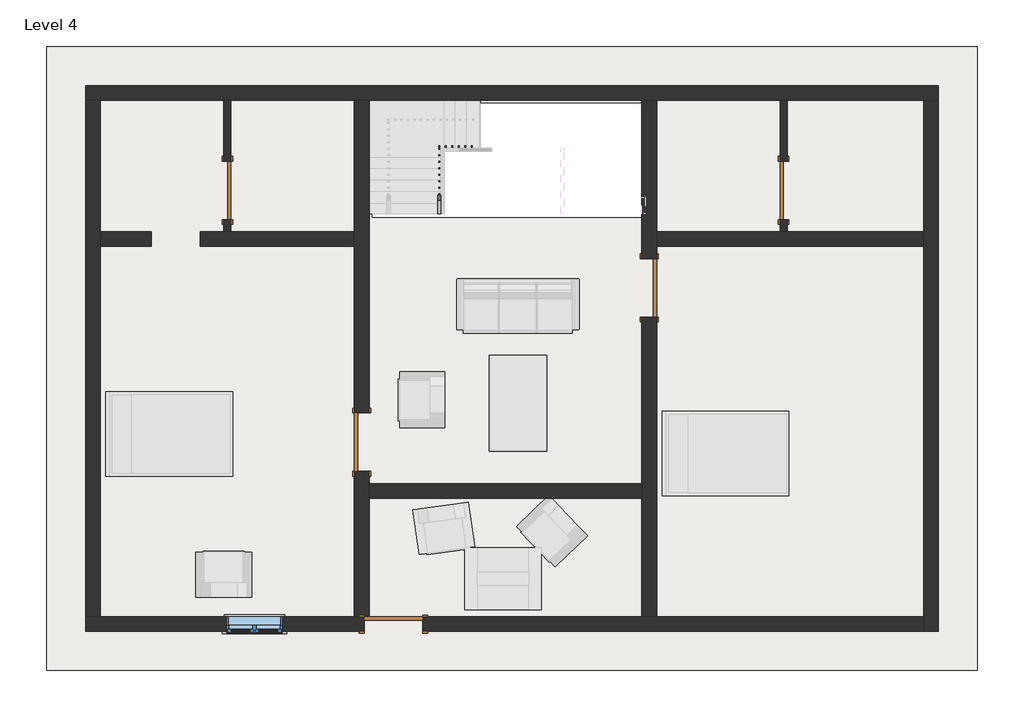
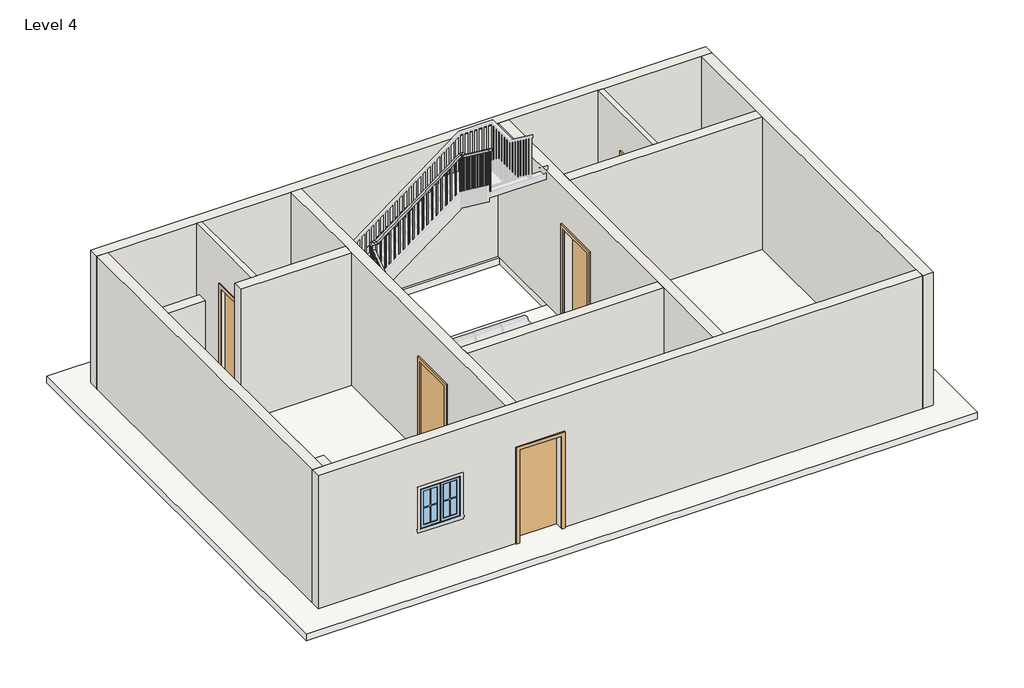
# One storey, part 1 of 2: 12 walls, 5 doors, 1 railing, 1 roof, 1 window.
"""IFC4 building model written with IfcOpenShell, lengths in millimetres."""

from ifc_helpers import new_model, si_unit, frame, origin, place, context, project, spatial, polyline, outline, extrude, faceted_brep, transform, mapped, element, save
from components import door_e5f9f3c4, door_a90ba1ad, door_305aa2a5, window_339605e1

model = new_model("IFC4")

# Units and contexts
model_context = context("Model", 3, world=origin())
ifc_project = project(units=[si_unit("LENGTHUNIT", "METRE", prefix="MILLI")], contexts=[model_context])

# Site, building, storey
site = spatial("IfcSite", under=ifc_project)
building = spatial("IfcBuilding", under=site)
storey = spatial("IfcBuildingStorey", under=building, Name="Level 4", Elevation=6400.8)

# Doors
placement = place(None, origin())
door_shape = door_e5f9f3c4(model_context)
element("IfcDoor", 1, ObjectType="Single-Flush : 36\" x 84\"", at=placement, inside=storey, context=model_context, shape_type="MappedRepresentation", body=[
    mapped(door_shape, transform((-5709.1546642, 5087.2167606, 6400.8), x_axis=(0.0, -1.0, 0.0), y_axis=(1.0, 0.0, 0.0), z_axis=(0.0, 0.0, 1.0))),
])
door_2_shape = door_a90ba1ad(model_context)
element("IfcDoor", 2, ObjectType="Single-Flush : 36\" x 84\"", at=placement, inside=storey, context=model_context, shape_type="MappedRepresentation", body=[
    mapped(door_2_shape, transform((-3607.3046642, 1150.2167606, 6400.8), x_axis=(0.0, -1.0, 0.0), y_axis=(1.0, 0.0, 0.0), z_axis=(0.0, 0.0, 1.0))),
])
element("IfcDoor", 3, ObjectType="Single-Flush : 36\" x 84\"", at=placement, inside=storey, context=model_context, shape_type="MappedRepresentation", body=[
    mapped(door_2_shape, transform((888.4953358, 3563.2167606, 6400.8), x_axis=(0.0, 1.0, 0.0), y_axis=(-1.0, 0.0, 0.0), z_axis=(0.0, 0.0, 1.0))),
])
element("IfcDoor", 4, ObjectType="Single-Flush : 36\" x 84\"", at=placement, inside=storey, context=model_context, shape_type="MappedRepresentation", body=[
    mapped(door_2_shape, transform((-3112.0046642, -1694.5832394, 6400.8), x_axis=(-1.0, 0.0, 0.0), y_axis=(0.0, -1.0, 0.0), z_axis=(0.0, 0.0, 1.0))),
])
door_3_shape = door_305aa2a5(model_context)
element("IfcDoor", 5, ObjectType="Single-Flush : 36\" x 84\"", at=placement, inside=storey, context=model_context, shape_type="MappedRepresentation", body=[
    mapped(door_3_shape, transform((2990.3453358, 5087.2167606, 6400.8), x_axis=(0.0, -1.0, 0.0), y_axis=(1.0, 0.0, 0.0), z_axis=(0.0, 0.0, 1.0))),
])

# Railing
element("IfcRailing", 6, ObjectType="Handrail - Rectangular", at=placement, inside=storey, context=model_context, shape_type="SolidModel", body=[
    faceted_brep([(-2419.4972892, 4718.9167606, 7447.7217391), (-2419.4972892, 4718.9167606, 7384.3634439), (-2368.6972892, 4718.9167606, 7384.3634439), (-2368.6972892, 4718.9167606, 7447.7217391), (-2419.4972892, 5670.3536537, 8156.8672495), (-2419.4972892, 5721.1536537, 8131.3723083), (-2368.6972892, 5721.1536537, 8131.3723083), (-2368.6972892, 5670.3536537, 8156.8672495), (-2419.4972892, 5670.3536537, 8263.6733611), (-2419.4972892, 5721.1536537, 8212.8733611), (-2368.6972892, 5721.1536537, 8212.8733611), (-2368.6972892, 5670.3536537, 8263.6733611), (-2419.4972892, 5797.3536537, 8263.6733611), (-2419.4972892, 5797.3536537, 8212.8733611), (-2368.6972892, 5746.5536537, 8212.8733611), (-2368.6972892, 5746.5536537, 8263.6733611), (-2292.4972892, 5797.3536537, 8263.6733611), (-2275.6482431, 5797.3536537, 8212.8733611), (-2275.6482431, 5746.5536537, 8212.8733611), (-2292.4972892, 5746.5536537, 8263.6733611), (-474.1369697, 5797.3536537, 9618.9729781), (-457.2879235, 5797.3536537, 9568.1729781), (-457.2879235, 5746.5536537, 9568.1729781), (-474.1369697, 5746.5536537, 9618.9729781), (-394.2046642, 5797.3536537, 9618.9729781), (-394.2046642, 5797.3536537, 9568.1729781), (-445.0046642, 5746.5536537, 9568.1729781), (-445.0046642, 5746.5536537, 9618.9729781), (-394.2046642, 5717.4213483, 9618.9729781), (-394.2046642, 5700.5723021, 9568.1729781), (-445.0046642, 5700.5723021, 9568.1729781), (-445.0046642, 5717.4213483, 9618.9729781), (-394.2046642, 4718.9167606, 10363.2), (-445.0046642, 4718.9167606, 10363.2), (-445.0046642, 4718.9167606, 10299.8417047), (-394.2046642, 4718.9167606, 10299.8417047)], [[[0, 1, 2, 3]], [[1, 0, 4, 5]], [[2, 1, 5, 6]], [[3, 2, 6, 7]], [[0, 3, 7, 4]], [[5, 4, 8, 9]], [[6, 5, 9, 10]], [[7, 6, 10, 11]], [[4, 7, 11, 8]], [[9, 8, 12, 13]], [[10, 9, 13, 14]], [[11, 10, 14, 15]], [[8, 11, 15, 12]], [[13, 12, 16, 17]], [[14, 13, 17, 18]], [[15, 14, 18, 19]], [[12, 15, 19, 16]], [[17, 16, 20, 21]], [[18, 17, 21, 22]], [[19, 18, 22, 23]], [[16, 19, 23, 20]], [[21, 20, 24, 25]], [[22, 21, 25, 26]], [[23, 22, 26, 27]], [[20, 23, 27, 24]], [[25, 24, 28, 29]], [[26, 25, 29, 30]], [[27, 26, 30, 31]], [[24, 27, 31, 28]], [[32, 33, 34, 35]], [[29, 28, 32, 35]], [[30, 29, 35, 34]], [[31, 30, 34, 33]], [[28, 31, 33, 32]]]),
    extrude(outline(polyline([(4746.4286537, 10279.3359459), (4765.4786537, 10265.1371882), (4765.4786537, 9316.2782609), (4746.4286537, 9316.2782609), (4746.4286537, 10279.3359459)])), frame((-429.1296642, 0.0, 0.0), z_axis=(1.0, 0.0, 0.0), x_axis=(0.0, 1.0, 0.0)), (0.0, 0.0, 1.0), 19.05),
    extrude(outline(polyline([(4848.0286537, 10203.6092378), (4867.0786537, 10189.4104801), (4867.0786537, 9316.2782609), (4848.0286537, 9316.2782609), (4848.0286537, 10203.6092378)])), frame((-429.1296642, 0.0, 0.0), z_axis=(1.0, 0.0, 0.0), x_axis=(0.0, 1.0, 0.0)), (0.0, 0.0, 1.0), 19.05),
    extrude(outline(polyline([(4949.6286537, 10127.8825298), (4968.6786537, 10113.683772), (4968.6786537, 9183.7565217), (4949.6286537, 9183.7565217), (4949.6286537, 10127.8825298)])), frame((-429.1296642, 0.0, 0.0), z_axis=(1.0, 0.0, 0.0), x_axis=(0.0, 1.0, 0.0)), (0.0, 0.0, 1.0), 19.05),
    extrude(outline(polyline([(5051.2286537, 10052.1558217), (5070.2786537, 10037.9570639), (5070.2786537, 9183.7565217), (5051.2286537, 9183.7565217), (5051.2286537, 10052.1558217)])), frame((-429.1296642, 0.0, 0.0), z_axis=(1.0, 0.0, 0.0), x_axis=(0.0, 1.0, 0.0)), (0.0, 0.0, 1.0), 19.05),
    extrude(outline(polyline([(5152.8286537, 9976.4291136), (5171.8786537, 9962.2303559), (5171.8786537, 9051.2347826), (5152.8286537, 9051.2347826), (5152.8286537, 9976.4291136)])), frame((-429.1296642, 0.0, 0.0), z_axis=(1.0, 0.0, 0.0), x_axis=(0.0, 1.0, 0.0)), (0.0, 0.0, 1.0), 19.05),
    extrude(outline(polyline([(5254.4286537, 9900.7024055), (5273.4786537, 9886.5036478), (5273.4786537, 8918.7130435), (5254.4286537, 8918.7130435), (5254.4286537, 9900.7024055)])), frame((-429.1296642, 0.0, 0.0), z_axis=(1.0, 0.0, 0.0), x_axis=(0.0, 1.0, 0.0)), (0.0, 0.0, 1.0), 19.05),
    extrude(outline(polyline([(5356.0286537, 9824.9756975), (5375.0786537, 9810.7769397), (5375.0786537, 8918.7130435), (5356.0286537, 8918.7130435), (5356.0286537, 9824.9756975)])), frame((-429.1296642, 0.0, 0.0), z_axis=(1.0, 0.0, 0.0), x_axis=(0.0, 1.0, 0.0)), (0.0, 0.0, 1.0), 19.05),
    extrude(outline(polyline([(5457.6286537, 9749.2489894), (5476.6786537, 9735.0502316), (5476.6786537, 8786.1913043), (5457.6286537, 8786.1913043), (5457.6286537, 9749.2489894)])), frame((-429.1296642, 0.0, 0.0), z_axis=(1.0, 0.0, 0.0), x_axis=(0.0, 1.0, 0.0)), (0.0, 0.0, 1.0), 19.05),
    extrude(outline(polyline([(5559.2286537, 9673.5222813), (5578.2786537, 9659.3235236), (5578.2786537, 8786.1913043), (5559.2286537, 8786.1913043), (5559.2286537, 9673.5222813)])), frame((-429.1296642, 0.0, 0.0), z_axis=(1.0, 0.0, 0.0), x_axis=(0.0, 1.0, 0.0)), (0.0, 0.0, 1.0), 19.05),
    extrude(outline(polyline([(5660.8286537, 9597.7955732), (5679.8786537, 9583.5968155), (5679.8786537, 8653.6695652), (5660.8286537, 8653.6695652), (5660.8286537, 9597.7955732)])), frame((-429.1296642, 0.0, 0.0), z_axis=(1.0, 0.0, 0.0), x_axis=(0.0, 1.0, 0.0)), (0.0, 0.0, 1.0), 19.05),
    extrude(outline(polyline([(-473.2222892, 5762.4286537), (-473.2222892, 5781.4786537), (-454.1722892, 5781.4786537), (-454.1722892, 5762.4286537), (-473.2222892, 5762.4286537)])), frame((0.0, 0.0, 8653.6695652), z_axis=(0.0, 0.0, 1.0), x_axis=(1.0, 0.0, 0.0)), (0.0, 0.0, 1.0), 914.5034129),
    extrude(outline(polyline([(9494.7684819, -555.7722892), (9480.5697242, -574.8222892), (8521.1478261, -574.8222892), (8521.1478261, -555.7722892), (9494.7684819, -555.7722892)])), frame((0.0, 5762.4286537, 0.0), z_axis=(0.0, 1.0, 0.0), x_axis=(0.0, 0.0, 1.0)), (0.0, 0.0, 1.0), 19.05),
    extrude(outline(polyline([(9419.0417739, -657.3722892), (9404.8430161, -676.4222892), (8521.1478261, -676.4222892), (8521.1478261, -657.3722892), (9419.0417739, -657.3722892)])), frame((0.0, 5762.4286537, 0.0), z_axis=(0.0, 1.0, 0.0), x_axis=(0.0, 0.0, 1.0)), (0.0, 0.0, 1.0), 19.05),
    extrude(outline(polyline([(9343.3150658, -758.9722892), (9329.116308, -778.0222892), (8388.626087, -778.0222892), (8388.626087, -758.9722892), (9343.3150658, -758.9722892)])), frame((0.0, 5762.4286537, 0.0), z_axis=(0.0, 1.0, 0.0), x_axis=(0.0, 0.0, 1.0)), (0.0, 0.0, 1.0), 19.05),
    extrude(outline(polyline([(9267.5883577, -860.5722892), (9253.3896, -879.6222892), (8388.626087, -879.6222892), (8388.626087, -860.5722892), (9267.5883577, -860.5722892)])), frame((0.0, 5762.4286537, 0.0), z_axis=(0.0, 1.0, 0.0), x_axis=(0.0, 0.0, 1.0)), (0.0, 0.0, 1.0), 19.05),
    extrude(outline(polyline([(9191.8616496, -962.1722892), (9177.6628919, -981.2222892), (8256.1043478, -981.2222892), (8256.1043478, -962.1722892), (9191.8616496, -962.1722892)])), frame((0.0, 5762.4286537, 0.0), z_axis=(0.0, 1.0, 0.0), x_axis=(0.0, 0.0, 1.0)), (0.0, 0.0, 1.0), 19.05),
    extrude(outline(polyline([(9116.1349416, -1063.7722892), (9101.9361838, -1082.8222892), (8256.1043478, -1082.8222892), (8256.1043478, -1063.7722892), (9116.1349416, -1063.7722892)])), frame((0.0, 5762.4286537, 0.0), z_axis=(0.0, 1.0, 0.0), x_axis=(0.0, 0.0, 1.0)), (0.0, 0.0, 1.0), 19.05),
    extrude(outline(polyline([(9040.4082335, -1165.3722892), (9026.2094757, -1184.4222892), (8123.5826087, -1184.4222892), (8123.5826087, -1165.3722892), (9040.4082335, -1165.3722892)])), frame((0.0, 5762.4286537, 0.0), z_axis=(0.0, 1.0, 0.0), x_axis=(0.0, 0.0, 1.0)), (0.0, 0.0, 1.0), 19.05),
    extrude(outline(polyline([(8964.6815254, -1266.9722892), (8950.4827677, -1286.0222892), (7991.0608696, -1286.0222892), (7991.0608696, -1266.9722892), (8964.6815254, -1266.9722892)])), frame((0.0, 5762.4286537, 0.0), z_axis=(0.0, 1.0, 0.0), x_axis=(0.0, 0.0, 1.0)), (0.0, 0.0, 1.0), 19.05),
    extrude(outline(polyline([(8888.9548173, -1368.5722892), (8874.7560596, -1387.6222892), (7991.0608696, -1387.6222892), (7991.0608696, -1368.5722892), (8888.9548173, -1368.5722892)])), frame((0.0, 5762.4286537, 0.0), z_axis=(0.0, 1.0, 0.0), x_axis=(0.0, 0.0, 1.0)), (0.0, 0.0, 1.0), 19.05),
    extrude(outline(polyline([(8813.2281093, -1470.1722892), (8799.0293515, -1489.2222892), (7858.5391304, -1489.2222892), (7858.5391304, -1470.1722892), (8813.2281093, -1470.1722892)])), frame((0.0, 5762.4286537, 0.0), z_axis=(0.0, 1.0, 0.0), x_axis=(0.0, 0.0, 1.0)), (0.0, 0.0, 1.0), 19.05),
    extrude(outline(polyline([(8737.5014012, -1571.7722892), (8723.3026434, -1590.8222892), (7858.5391304, -1590.8222892), (7858.5391304, -1571.7722892), (8737.5014012, -1571.7722892)])), frame((0.0, 5762.4286537, 0.0), z_axis=(0.0, 1.0, 0.0), x_axis=(0.0, 0.0, 1.0)), (0.0, 0.0, 1.0), 19.05),
    extrude(outline(polyline([(8661.7746931, -1673.3722892), (8647.5759354, -1692.4222892), (7726.0173913, -1692.4222892), (7726.0173913, -1673.3722892), (8661.7746931, -1673.3722892)])), frame((0.0, 5762.4286537, 0.0), z_axis=(0.0, 1.0, 0.0), x_axis=(0.0, 0.0, 1.0)), (0.0, 0.0, 1.0), 19.05),
    extrude(outline(polyline([(8586.047985, -1774.9722892), (8571.8492273, -1794.0222892), (7726.0173913, -1794.0222892), (7726.0173913, -1774.9722892), (8586.047985, -1774.9722892)])), frame((0.0, 5762.4286537, 0.0), z_axis=(0.0, 1.0, 0.0), x_axis=(0.0, 0.0, 1.0)), (0.0, 0.0, 1.0), 19.05),
    extrude(outline(polyline([(8510.321277, -1876.5722892), (8496.1225192, -1895.6222892), (7593.4956522, -1895.6222892), (7593.4956522, -1876.5722892), (8510.321277, -1876.5722892)])), frame((0.0, 5762.4286537, 0.0), z_axis=(0.0, 1.0, 0.0), x_axis=(0.0, 0.0, 1.0)), (0.0, 0.0, 1.0), 19.05),
    extrude(outline(polyline([(8434.5945689, -1978.1722892), (8420.3958111, -1997.2222892), (7460.973913, -1997.2222892), (7460.973913, -1978.1722892), (8434.5945689, -1978.1722892)])), frame((0.0, 5762.4286537, 0.0), z_axis=(0.0, 1.0, 0.0), x_axis=(0.0, 0.0, 1.0)), (0.0, 0.0, 1.0), 19.05),
    extrude(outline(polyline([(8358.8678608, -2079.7722892), (8344.6691031, -2098.8222892), (7460.973913, -2098.8222892), (7460.973913, -2079.7722892), (8358.8678608, -2079.7722892)])), frame((0.0, 5762.4286537, 0.0), z_axis=(0.0, 1.0, 0.0), x_axis=(0.0, 0.0, 1.0)), (0.0, 0.0, 1.0), 19.05),
    extrude(outline(polyline([(8283.1411527, -2181.3722892), (8268.942395, -2200.4222892), (7328.4521739, -2200.4222892), (7328.4521739, -2181.3722892), (8283.1411527, -2181.3722892)])), frame((0.0, 5762.4286537, 0.0), z_axis=(0.0, 1.0, 0.0), x_axis=(0.0, 0.0, 1.0)), (0.0, 0.0, 1.0), 19.05),
    extrude(outline(polyline([(8207.4144447, -2282.9722892), (8193.2156869, -2302.0222892), (7328.4521739, -2302.0222892), (7328.4521739, -2282.9722892), (8207.4144447, -2282.9722892)])), frame((0.0, 5762.4286537, 0.0), z_axis=(0.0, 1.0, 0.0), x_axis=(0.0, 0.0, 1.0)), (0.0, 0.0, 1.0), 19.05),
    extrude(outline(polyline([(-2384.5722892, 5725.3917606), (-2403.6222892, 5725.3917606), (-2403.6222892, 5744.4417606), (-2384.5722892, 5744.4417606), (-2384.5722892, 5725.3917606)])), frame((0.0, 0.0, 7195.9304348), z_axis=(0.0, 0.0, 1.0), x_axis=(1.0, 0.0, 0.0)), (0.0, 0.0, 1.0), 1016.9429263),
    extrude(outline(polyline([(5623.7917606, 8058.8044377), (5642.8417606, 8073.0031954), (5642.8417606, 7195.9304348), (5623.7917606, 7195.9304348), (5623.7917606, 8058.8044377)])), frame((-2403.6222892, 0.0, 0.0), z_axis=(1.0, 0.0, 0.0), x_axis=(0.0, 1.0, 0.0)), (0.0, 0.0, 1.0), 19.05),
    extrude(outline(polyline([(5522.1917606, 7983.0777296), (5541.2417606, 7997.2764873), (5541.2417606, 7063.4086957), (5522.1917606, 7063.4086957), (5522.1917606, 7983.0777296)])), frame((-2403.6222892, 0.0, 0.0), z_axis=(1.0, 0.0, 0.0), x_axis=(0.0, 1.0, 0.0)), (0.0, 0.0, 1.0), 19.05),
    extrude(outline(polyline([(5420.5917606, 7907.3510215), (5439.6417606, 7921.5497793), (5439.6417606, 7063.4086957), (5420.5917606, 7063.4086957), (5420.5917606, 7907.3510215)])), frame((-2403.6222892, 0.0, 0.0), z_axis=(1.0, 0.0, 0.0), x_axis=(0.0, 1.0, 0.0)), (0.0, 0.0, 1.0), 19.05),
    extrude(outline(polyline([(5318.9917606, 7831.6243134), (5338.0417606, 7845.8230712), (5338.0417606, 6930.8869565), (5318.9917606, 6930.8869565), (5318.9917606, 7831.6243134)])), frame((-2403.6222892, 0.0, 0.0), z_axis=(1.0, 0.0, 0.0), x_axis=(0.0, 1.0, 0.0)), (0.0, 0.0, 1.0), 19.05),
    extrude(outline(polyline([(5217.3917606, 7755.8976054), (5236.4417606, 7770.0963631), (5236.4417606, 6798.3652174), (5217.3917606, 6798.3652174), (5217.3917606, 7755.8976054)])), frame((-2403.6222892, 0.0, 0.0), z_axis=(1.0, 0.0, 0.0), x_axis=(0.0, 1.0, 0.0)), (0.0, 0.0, 1.0), 19.05),
    extrude(outline(polyline([(5115.7917606, 7680.1708973), (5134.8417606, 7694.369655), (5134.8417606, 6798.3652174), (5115.7917606, 6798.3652174), (5115.7917606, 7680.1708973)])), frame((-2403.6222892, 0.0, 0.0), z_axis=(1.0, 0.0, 0.0), x_axis=(0.0, 1.0, 0.0)), (0.0, 0.0, 1.0), 19.05),
    extrude(outline(polyline([(5014.1917606, 7604.4441892), (5033.2417606, 7618.642947), (5033.2417606, 6665.8434783), (5014.1917606, 6665.8434783), (5014.1917606, 7604.4441892)])), frame((-2403.6222892, 0.0, 0.0), z_axis=(1.0, 0.0, 0.0), x_axis=(0.0, 1.0, 0.0)), (0.0, 0.0, 1.0), 19.05),
    extrude(outline(polyline([(4912.5917606, 7528.7174811), (4931.6417606, 7542.9162389), (4931.6417606, 6665.8434783), (4912.5917606, 6665.8434783), (4912.5917606, 7528.7174811)])), frame((-2403.6222892, 0.0, 0.0), z_axis=(1.0, 0.0, 0.0), x_axis=(0.0, 1.0, 0.0)), (0.0, 0.0, 1.0), 19.05),
    extrude(outline(polyline([(4810.9917606, 7452.9907731), (4830.0417606, 7467.1895308), (4830.0417606, 6533.3217391), (4810.9917606, 6533.3217391), (4810.9917606, 7452.9907731)])), frame((-2403.6222892, 0.0, 0.0), z_axis=(1.0, 0.0, 0.0), x_axis=(0.0, 1.0, 0.0)), (0.0, 0.0, 1.0), 19.05),
    extrude(outline(polyline([(-429.1296642, 5762.4286537), (-429.1296642, 5781.4786537), (-410.0796642, 5781.4786537), (-410.0796642, 5762.4286537), (-429.1296642, 5762.4286537)])), frame((0.0, 0.0, 8653.6695652), z_axis=(0.0, 0.0, 1.0), x_axis=(1.0, 0.0, 0.0)), (0.0, 0.0, 1.0), 914.5034129),
    extrude(outline(polyline([(-2384.5722892, 5762.4286537), (-2403.6222892, 5762.4286537), (-2403.6222892, 5781.4786537), (-2384.5722892, 5781.4786537), (-2384.5722892, 5762.4286537)])), frame((0.0, 0.0, 7195.9304348), z_axis=(0.0, 0.0, 1.0), x_axis=(1.0, 0.0, 0.0)), (0.0, 0.0, 1.0), 1016.9429263),
    extrude(outline(polyline([(4718.9167606, 10299.8417047), (4737.9667606, 10285.642947), (4737.9667606, 9316.2782609), (4718.9167606, 9316.2782609), (4718.9167606, 10299.8417047)])), frame((-429.1296642, 0.0, 0.0), z_axis=(1.0, 0.0, 0.0), x_axis=(0.0, 1.0, 0.0)), (0.0, 0.0, 1.0), 19.05),
    extrude(outline(polyline([(4718.9167606, 7384.3634439), (4737.9667606, 7398.5622016), (4737.9667606, 6533.3217391), (4718.9167606, 6533.3217391), (4718.9167606, 7384.3634439)])), frame((-2403.6222892, 0.0, 0.0), z_axis=(1.0, 0.0, 0.0), x_axis=(0.0, 1.0, 0.0)), (0.0, 0.0, 1.0), 19.05),
])

# Roof
element("IfcRoof", 7, ObjectType="Generic - 12\"", at=placement, inside=storey, context=model_context, shape_type="SweptSolid", body=[
    extrude(outline(polyline([(6019.2953358, 7335.1167606), (6019.2953358, -2418.4832394), (-8534.9046642, -2418.4832394), (-8534.9046642, 7335.1167606), (6019.2953358, 7335.1167606)]), holes=[polyline([(774.1953358, 6446.1167606), (-3442.2046642, 6446.1167606), (-3442.2046642, 4668.1167606), (774.1953358, 4668.1167606), (774.1953358, 6446.1167606)])]), frame((0.0, 0.0, 6248.4), z_axis=(0.0, 0.0, 1.0), x_axis=(1.0, 0.0, 0.0)), (0.0, 0.0, 1.0), 152.4),
])

# Walls
element("IfcWall", 8, ObjectType="WALL4.5\"", at=placement, inside=storey, context=model_context, shape_type="SweptSolid", body=[
    extrude(outline(polyline([(4630.0167606, 8534.4), (4630.0167606, 6400.8), (4439.5167606, 6400.8), (4439.5167606, 9448.8), (6496.9167606, 9448.8), (6496.9167606, 6400.8), (5544.4167606, 6400.8), (5544.4167606, 8534.4), (4630.0167606, 8534.4)])), frame((-5766.3046642, 0.0, 0.0), z_axis=(1.0, 0.0, 0.0), x_axis=(0.0, 1.0, 0.0)), (0.0, 0.0, 1.0), 114.3),
])
element("IfcWall", 9, ObjectType="WALL4.5\"", at=placement, inside=storey, context=model_context, shape_type="SweptSolid", body=[
    extrude(outline(polyline([(4630.0167606, 8534.4), (4630.0167606, 6400.8), (4439.5167606, 6400.8), (4439.5167606, 9448.8), (6496.9167606, 9448.8), (6496.9167606, 6400.8), (5544.4167606, 6400.8), (5544.4167606, 8534.4), (4630.0167606, 8534.4)])), frame((2933.1953358, 0.0, 0.0), z_axis=(1.0, 0.0, 0.0), x_axis=(0.0, 1.0, 0.0)), (0.0, 0.0, 1.0), 114.3),
])
element("IfcWall", 10, ObjectType="WALL9\"", at=placement, inside=storey, context=model_context, shape_type="Brep", body=[
    faceted_brep([(-7925.3046642, 6496.9167606, 6400.8), (-7696.7046642, 6496.9167606, 6400.8), (-5766.3046642, 6496.9167606, 6400.8), (-5652.0046642, 6496.9167606, 6400.8), (-3721.6046642, 6496.9167606, 6400.8), (-3493.0046642, 6496.9167606, 6400.8), (774.1953358, 6496.9167606, 6400.8), (1002.7953358, 6496.9167606, 6400.8), (2933.1953358, 6496.9167606, 6400.8), (3047.4953358, 6496.9167606, 6400.8), (5181.0953358, 6496.9167606, 6400.8), (5409.6953358, 6496.9167606, 6400.8), (5409.6953358, 6496.9167606, 9448.8), (5181.0953358, 6496.9167606, 9448.8), (3047.4953358, 6496.9167606, 9448.8), (2933.1953358, 6496.9167606, 9448.8), (1002.7953358, 6496.9167606, 9448.8), (774.1953358, 6496.9167606, 9448.8), (-3493.0046642, 6496.9167606, 9448.8), (-3721.6046642, 6496.9167606, 9448.8), (-5652.0046642, 6496.9167606, 9448.8), (-5766.3046642, 6496.9167606, 9448.8), (-7696.7046642, 6496.9167606, 9448.8), (-7925.3046642, 6496.9167606, 9448.8), (-7925.3046642, 6725.5167606, 6400.8), (-7925.3046642, 6725.5167606, 9448.8), (5409.6953358, 6725.5167606, 9448.8), (5409.6953358, 6725.5167606, 6400.8)], [[[0, 1, 2, 3, 4, 5, 6, 7, 8, 9, 10, 11, 12, 13, 14, 15, 16, 17, 18, 19, 20, 21, 22, 23]], [[24, 25, 26, 27]], [[11, 10, 9, 8, 7, 6, 5, 4, 3, 2, 1, 0, 24, 27]], [[12, 11, 27, 26]], [[0, 23, 25, 24]], [[23, 22, 21, 20, 19, 18, 17, 16, 15, 14, 13, 12, 26, 25]]]),
])
element("IfcWall", 11, ObjectType="WALL9\"", at=placement, inside=storey, context=model_context, shape_type="Brep", body=[
    faceted_brep([(5181.0953358, 6496.9167606, 6400.8), (5181.0953358, 4439.5167606, 6400.8), (5181.0953358, 4210.9167606, 6400.8), (5181.0953358, -1580.2832394, 6400.8), (5181.0953358, -1808.8832394, 6400.8), (5181.0953358, -1808.8832394, 9448.8), (5181.0953358, -1580.2832394, 9448.8), (5181.0953358, 4210.9167606, 9448.8), (5181.0953358, 4439.5167606, 9448.8), (5181.0953358, 6496.9167606, 9448.8), (5409.6953358, 6496.9167606, 6400.8), (5409.6953358, 6496.9167606, 9448.8), (5409.6953358, -1808.8832394, 9448.8), (5409.6953358, -1808.8832394, 6400.8)], [[[0, 1, 2, 3, 4, 5, 6, 7, 8, 9]], [[10, 11, 12, 13]], [[4, 3, 2, 1, 0, 10, 13]], [[0, 9, 11, 10]], [[5, 4, 13, 12]], [[9, 8, 7, 6, 5, 12, 11]]]),
])
element("IfcWall", 12, ObjectType="WALL9\"", at=placement, inside=storey, context=model_context, shape_type="Brep", body=[
    faceted_brep([(-3569.2046642, -1580.2832394, 8534.4), (-3569.2046642, -1580.2832394, 6400.8), (-3721.6046642, -1580.2832394, 6400.8), (-7696.7046642, -1580.2832394, 6400.8), (-7925.3046642, -1580.2832394, 6400.8), (-7925.3046642, -1580.2832394, 9448.8), (-7696.7046642, -1580.2832394, 9448.8), (-3721.6046642, -1580.2832394, 9448.8), (-3493.0046642, -1580.2832394, 9448.8), (774.1953358, -1580.2832394, 9448.8), (1002.7953358, -1580.2832394, 9448.8), (5181.0953358, -1580.2832394, 9448.8), (5181.0953358, -1580.2832394, 6400.8), (1002.7953358, -1580.2832394, 6400.8), (774.1953358, -1580.2832394, 6400.8), (-2654.8046642, -1580.2832394, 6400.8), (-2654.8046642, -1580.2832394, 8534.4), (-5715.5046642, -1580.2832394, 8382.3434313), (-5715.5046642, -1580.2832394, 7467.9434313), (-4851.9046642, -1580.2832394, 7467.9434313), (-4851.9046642, -1580.2832394, 8382.3434313), (-7925.3046642, -1808.8832394, 6400.8), (-3569.2046642, -1808.8832394, 6400.8), (-3569.2046642, -1808.8832394, 8534.4), (-2654.8046642, -1808.8832394, 8534.4), (-2654.8046642, -1808.8832394, 6400.8), (5181.0953358, -1808.8832394, 6400.8), (5181.0953358, -1808.8832394, 9448.8), (-7925.3046642, -1808.8832394, 9448.8), (-5715.5046642, -1808.8832394, 8382.3434313), (-4851.9046642, -1808.8832394, 8382.3434313), (-4851.9046642, -1808.8832394, 7467.9434313), (-5715.5046642, -1808.8832394, 7467.9434313)], [[[0, 1, 2, 3, 4, 5, 6, 7, 8, 9, 10, 11, 12, 13, 14, 15, 16], [17, 18, 19, 20]], [[21, 22, 23, 24, 25, 26, 27, 28], [29, 30, 31, 32]], [[4, 3, 2, 1, 22, 21]], [[15, 14, 13, 12, 26, 25]], [[12, 11, 27, 26]], [[5, 4, 21, 28]], [[23, 22, 1, 0]], [[24, 23, 0, 16]], [[25, 24, 16, 15]], [[11, 10, 9, 8, 7, 6, 5, 28, 27]], [[18, 17, 29, 32]], [[19, 18, 32, 31]], [[20, 19, 31, 30]], [[17, 20, 30, 29]]]),
])
element("IfcWall", 13, ObjectType="WALL9\"", at=placement, inside=storey, context=model_context, shape_type="Brep", body=[
    faceted_brep([(-7696.7046642, -1580.2832394, 6400.8), (-7696.7046642, 4210.9167606, 6400.8), (-7696.7046642, 4439.5167606, 6400.8), (-7696.7046642, 6496.9167606, 6400.8), (-7696.7046642, 6496.9167606, 9448.8), (-7696.7046642, 4439.5167606, 9448.8), (-7696.7046642, 4210.9167606, 9448.8), (-7696.7046642, -1580.2832394, 9448.8), (-7925.3046642, -1580.2832394, 6400.8), (-7925.3046642, -1580.2832394, 9448.8), (-7925.3046642, 6496.9167606, 9448.8), (-7925.3046642, 6496.9167606, 6400.8)], [[[0, 1, 2, 3, 4, 5, 6, 7]], [[8, 9, 10, 11]], [[3, 2, 1, 0, 8, 11]], [[4, 3, 11, 10]], [[0, 7, 9, 8]], [[7, 6, 5, 4, 10, 9]]]),
])
element("IfcWall", 14, ObjectType="WALL9\"", at=placement, inside=storey, context=model_context, shape_type="Brep", body=[
    faceted_brep([(-3721.6046642, 693.0167606, 8534.4), (-3721.6046642, 693.0167606, 6400.8), (-3721.6046642, -1580.2832394, 6400.8), (-3721.6046642, -1580.2832394, 9448.8), (-3721.6046642, 4210.9167606, 9448.8), (-3721.6046642, 4439.5167606, 9448.8), (-3721.6046642, 6496.9167606, 9448.8), (-3721.6046642, 6496.9167606, 6400.8), (-3721.6046642, 4439.5167606, 6400.8), (-3721.6046642, 4210.9167606, 6400.8), (-3721.6046642, 1607.4167606, 6400.8), (-3721.6046642, 1607.4167606, 8534.4), (-3493.0046642, -1580.2832394, 6400.8), (-3493.0046642, 273.9167606, 6400.8), (-3493.0046642, 502.5167606, 6400.8), (-3493.0046642, 693.0167606, 6400.8), (-3493.0046642, 693.0167606, 8534.4), (-3493.0046642, 1607.4167606, 8534.4), (-3493.0046642, 1607.4167606, 6400.8), (-3493.0046642, 6496.9167606, 6400.8), (-3493.0046642, 6496.9167606, 9448.8), (-3493.0046642, 502.5167606, 9448.8), (-3493.0046642, 273.9167606, 9448.8), (-3493.0046642, -1580.2832394, 9448.8), (-3569.2046642, -1580.2832394, 6400.8)], [[[0, 1, 2, 3, 4, 5, 6, 7, 8, 9, 10, 11]], [[12, 13, 14, 15, 16, 17, 18, 19, 20, 21, 22, 23]], [[2, 1, 15, 14, 13, 12, 24]], [[10, 9, 8, 7, 19, 18]], [[7, 6, 20, 19]], [[3, 2, 24, 12, 23]], [[16, 15, 1, 0]], [[17, 16, 0, 11]], [[18, 17, 11, 10]], [[6, 5, 4, 3, 23, 22, 21, 20]]]),
])
element("IfcWall", 15, ObjectType="WALL9\"", at=placement, inside=storey, context=model_context, shape_type="Brep", body=[
    faceted_brep([(774.1953358, 6496.9167606, 6400.8), (774.1953358, 4020.4167606, 6400.8), (774.1953358, 4020.4167606, 8534.4), (774.1953358, 3106.0167606, 8534.4), (774.1953358, 3106.0167606, 6400.8), (774.1953358, 502.5167606, 6400.8), (774.1953358, 273.9167606, 6400.8), (774.1953358, -1580.2832394, 6400.8), (774.1953358, -1580.2832394, 9448.8), (774.1953358, 273.9167606, 9448.8), (774.1953358, 502.5167606, 9448.8), (774.1953358, 6496.9167606, 9448.8), (1002.7953358, 4020.4167606, 8534.4), (1002.7953358, 4020.4167606, 6400.8), (1002.7953358, 4210.9167606, 6400.8), (1002.7953358, 4439.5167606, 6400.8), (1002.7953358, 6496.9167606, 6400.8), (1002.7953358, 6496.9167606, 9448.8), (1002.7953358, 4439.5167606, 9448.8), (1002.7953358, 4210.9167606, 9448.8), (1002.7953358, -1580.2832394, 9448.8), (1002.7953358, -1580.2832394, 6400.8), (1002.7953358, 3106.0167606, 6400.8), (1002.7953358, 3106.0167606, 8534.4)], [[[0, 1, 2, 3, 4, 5, 6, 7, 8, 9, 10, 11]], [[12, 13, 14, 15, 16, 17, 18, 19, 20, 21, 22, 23]], [[22, 21, 7, 6, 5, 4]], [[16, 15, 14, 13, 1, 0]], [[0, 11, 17, 16]], [[8, 7, 21, 20]], [[2, 1, 13, 12]], [[3, 2, 12, 23]], [[4, 3, 23, 22]], [[11, 10, 9, 8, 20, 19, 18, 17]]]),
])
element("IfcWall", 16, ObjectType="WALL9\"", at=placement, inside=storey, context=model_context, shape_type="SweptSolid", body=[
    extrude(outline(polyline([(774.1953358, 273.9167606), (-3493.0046642, 273.9167606), (-3493.0046642, 502.5167606), (774.1953358, 502.5167606), (774.1953358, 273.9167606)])), frame((0.0, 0.0, 6400.8), z_axis=(0.0, 0.0, 1.0), x_axis=(1.0, 0.0, 0.0)), (0.0, 0.0, 1.0), 3048.0),
])
element("IfcWall", 17, ObjectType="WALL9\"", at=placement, inside=storey, context=model_context, shape_type="SweptSolid", body=[
    extrude(outline(polyline([(-6895.4507894, 4210.9167606), (-7696.7046642, 4210.9167606), (-7696.7046642, 4439.5167606), (-6895.4507894, 4439.5167606), (-6895.4507894, 4210.9167606)])), frame((0.0, 0.0, 6400.8), z_axis=(0.0, 0.0, 1.0), x_axis=(1.0, 0.0, 0.0)), (0.0, 0.0, 1.0), 3048.0),
])
element("IfcWall", 18, ObjectType="WALL9\"", at=placement, inside=storey, context=model_context, shape_type="Brep", body=[
    faceted_brep([(-3721.6046642, 4439.5167606, 6400.8), (-5652.0046642, 4439.5167606, 6400.8), (-5766.3046642, 4439.5167606, 6400.8), (-6131.0963491, 4439.5167606, 6400.8), (-6131.0963491, 4439.5167606, 9448.8), (-5766.3046642, 4439.5167606, 9448.8), (-5652.0046642, 4439.5167606, 9448.8), (-3721.6046642, 4439.5167606, 9448.8), (-3721.6046642, 4210.9167606, 6400.8), (-3721.6046642, 4210.9167606, 9448.8), (-6131.0963491, 4210.9167606, 9448.8), (-6131.0963491, 4210.9167606, 6400.8)], [[[0, 1, 2, 3, 4, 5, 6, 7]], [[8, 9, 10, 11]], [[3, 2, 1, 0, 8, 11]], [[4, 3, 11, 10]], [[0, 7, 9, 8]], [[7, 6, 5, 4, 10, 9]]]),
])
element("IfcWall", 19, ObjectType="WALL9\"", at=placement, inside=storey, context=model_context, shape_type="Brep", body=[
    faceted_brep([(1002.7953358, 4210.9167606, 6400.8), (5181.0953358, 4210.9167606, 6400.8), (5181.0953358, 4210.9167606, 9448.8), (1002.7953358, 4210.9167606, 9448.8), (1002.7953358, 4439.5167606, 6400.8), (1002.7953358, 4439.5167606, 9448.8), (2933.1953358, 4439.5167606, 9448.8), (3047.4953358, 4439.5167606, 9448.8), (5181.0953358, 4439.5167606, 9448.8), (5181.0953358, 4439.5167606, 6400.8), (3047.4953358, 4439.5167606, 6400.8), (2933.1953358, 4439.5167606, 6400.8)], [[[0, 1, 2, 3]], [[4, 5, 6, 7, 8, 9, 10, 11]], [[1, 0, 4, 11, 10, 9]], [[2, 1, 9, 8]], [[0, 3, 5, 4]], [[3, 2, 8, 7, 6, 5]]]),
])

# Window
window_shape = window_339605e1(model_context)
element("IfcWindow", 20, ObjectType="Window-Casement-Double : 34\" x 36\"", at=placement, inside=storey, context=model_context, shape_type="MappedRepresentation", body=[
    mapped(window_shape, transform((-5283.7046642, -1694.5832394, 6553.5434313), x_axis=(-1.0, 0.0, 0.0), y_axis=(0.0, -1.0, 0.0), z_axis=(0.0, 0.0, 1.0))),
])

save(model, "model.ifc")

# Revit data of these elements
# Type "Single-Flush : 36\" x 84\""
#   Type Mark = "1"
#   Construction Type Id = "MDOOR"
#   Assembly Code = "C1020"
#   Analytic Construction = "Metal"
#   Thickness = 0' - 2"
#   Heat Transfer Coefficient (U) = 0.651978 BTU/(h·ft²·°F)
#   Height = 7' - 0"
#   Trim Projection Ext = 0' - 1"
#   Trim Projection Int = 0' - 1"
#   Trim Width = 0' - 3"
#   Width = 3' - 0"
#   Define Thermal Properties by = 1
#   Define Thermal Properties by = 1
#   Door Material = Door - Panel
#   Frame Material = Door - Frame
#   Visual Light Transmittance = 0
#   Solar Heat Gain Coefficient = 0
#   Function = (empty or 0)
#   Wall Closure = (empty or 0)
# Type "Handrail - Rectangular"
#   Assembly Code = "C2010400"
#   built-in parameter 1008612 = 0.0416667 (stored number, unit not read)
#   built-in parameter 1008611 = 0.0416667 (stored number, unit not read)
#   built-in parameter 1008609 = 0.333333 (stored number, unit not read)
#   built-in parameter 1008604 = 0.166667 (stored number, unit not read)
#   built-in parameter 1008603 = 0.166667 (stored number, unit not read)
#   Railing Height = 3' - 0"
#   built-in parameter 1008630 = 2
#   built-in parameter 1008610 = 2
#   built-in parameter 1008618 = Baluster - Square : 3/4"
# Type "Generic - 12\""
#   Assembly Code = "B1020"
#   Layers, outside or top first: 0' - 6" no material (function 1)
# Type "WALL4.5\""
#   Assembly Code = "B2010"
#   Layers, outside or top first: 0' - 4 1/2" no material (function 1)
# Type "WALL9\""
#   Assembly Code = "B2010"
#   Layers, outside or top first: 0' - 9" no material (function 1)
# Type "Window-Casement-Double : 34\" x 36\""
#   Type Mark = "14"
#   Fire Rating = "0.5h"
#   Assembly Code = "B2020100"
#   Analytic Construction = "Double glazing - domestic"
#   Frame Extension [instance default] = 0' - 0 1/4"
#   Window Inset [instance default] = 0' - 0"
#   Wall Thickness [instance default] = 0' - 6"
#   Interior Wall Closure [instance default] = 0' - 2 1/4"
#   Half Width = 1' - 5"
#   Visual Light Transmittance = 0.81
#   Thermal Resistance (R) = 1.8146 (h·ft²·°F)/BTU
#   Solar Heat Gain Coefficient = 0.76
#   Rough Width = 2' - 10 1/2"
#   Rough Height = 3' - 0 1/2"
#   Height = 3' - 0"
#   Heat Transfer Coefficient (U) = 0.5511 BTU/(h·ft²·°F)
#   Exterior Wall Closure [instance default] = 0' - 1 1/4"
#   Extension Jamb [instance default] = 0' - 2 1/4"
#   Default Sill Height = 3' - 0"
#   Width = 2' - 10"
#   Define Thermal Properties by = 0
#   Muntin Visibility = yes
#   Interior Trim Visibility [instance default] = yes
#   Exterior Trim Visibility [instance default] = yes
#   Extension Jamb Visibility [instance default] = yes
#   Interior Trim Material = Wood - Stained
#   Muntin Pattern = Muntin Pattern_2x2 : Muntin Pattern_2x2
#   Interior Trim = Trim-Window-Interior-Flat : Picture Frame
#   Interior Frame Material = Wood - Stained
#   Glass Panel Material = Glass
#   Exterior Trim Material = Clad - White
#   Exterior Trim = Trim-Window-Exterior-Flat : with Sill
#   Exterior Frame Material = Clad - White
#   Wall Closure = (empty or 0)
# Elements 1, 2, 3, 4, 5 (IfcDoor, "Single-Flush : 36\" x 84\"")
#   Phase Created = New Construction
#   Materials on its faces: "Door - Frame", "Door - Panel"
# Element 6 (IfcRailing, "Handrail - Rectangular")
#   Phase Created = New Construction
# Element 7 (IfcRoof, "Generic - 12\"")
#   built-in parameter 1001705 = 21 (stored number, unit not read)
#   built-in parameter 1001701 = -0.5 (stored number, unit not read)
#   built-in parameter 1001710 = 33615
#   Phase Created = New Construction
#   Materials on its faces: "Default Roof", "TTT"
# Elements 8, 9 (IfcWall, "WALL4.5\"")
#   Top Offset = 0' - 0"
#   Base Offset = 0' - 0"
#   Unconnected Height = 10' - 0"
#   wall height = 10' - 0"
#   Phase Created = New Construction
#   Base Constraint = Level 4
#   Materials on its faces: "Default Wall"
# Elements 10, 11, 12, 13, 14, 15, 16, 17, 18, 19 (IfcWall, "WALL9\"")
#   Top Offset = 0' - 0"
#   Base Offset = 0' - 0"
#   Unconnected Height = 10' - 0"
#   wall height = 10' - 0"
#   Phase Created = New Construction
#   Base Constraint = Level 4
#   Materials on its faces: "Default Wall"
# Element 20 (IfcWindow, "Window-Casement-Double : 34\" x 36\"")
#   Mark = "3"
#   Window Inset = 0' - 0"
#   Interior Wall Closure = 0' - 2 1/4"
#   Frame Extension = 0' - 0 1/4"
#   Exterior Wall Closure = 0' - 1 1/4"
#   Interior Trim Visibility = yes
#   Exterior Trim Visibility = yes
#   Phase Created = New Construction
#   Materials on its faces: "Wood - Stained", "Glass", "Clad - White"
# Materials
#   "Door - Panel": class "Wood", colour RGB 210 159 95, transparency 0, Cost = 0
#   "Door - Frame": colour RGB 118 70 51, transparency 0, Cost = 0
#   "Wood - Stained": class "Wood", colour RGB 224 178 126, transparency 0, Cost = 0
#   "Glass": class "Glass", colour RGB 0 128 192, transparency 0.75, Description = "Soda Lime Glass", Cost = 0
#   "Clad - White": class "Wood", colour RGB 242 242 238, transparency 0, Cost = 0
#   "Default Roof": colour RGB 88 101 114, transparency 0, Cost = 0
#   "TTT": class "Generic", colour RGB 120 120 120, transparency 0, Cost = 0
#   "Default Wall": colour RGB 128 128 128, transparency 0, Cost = 0
